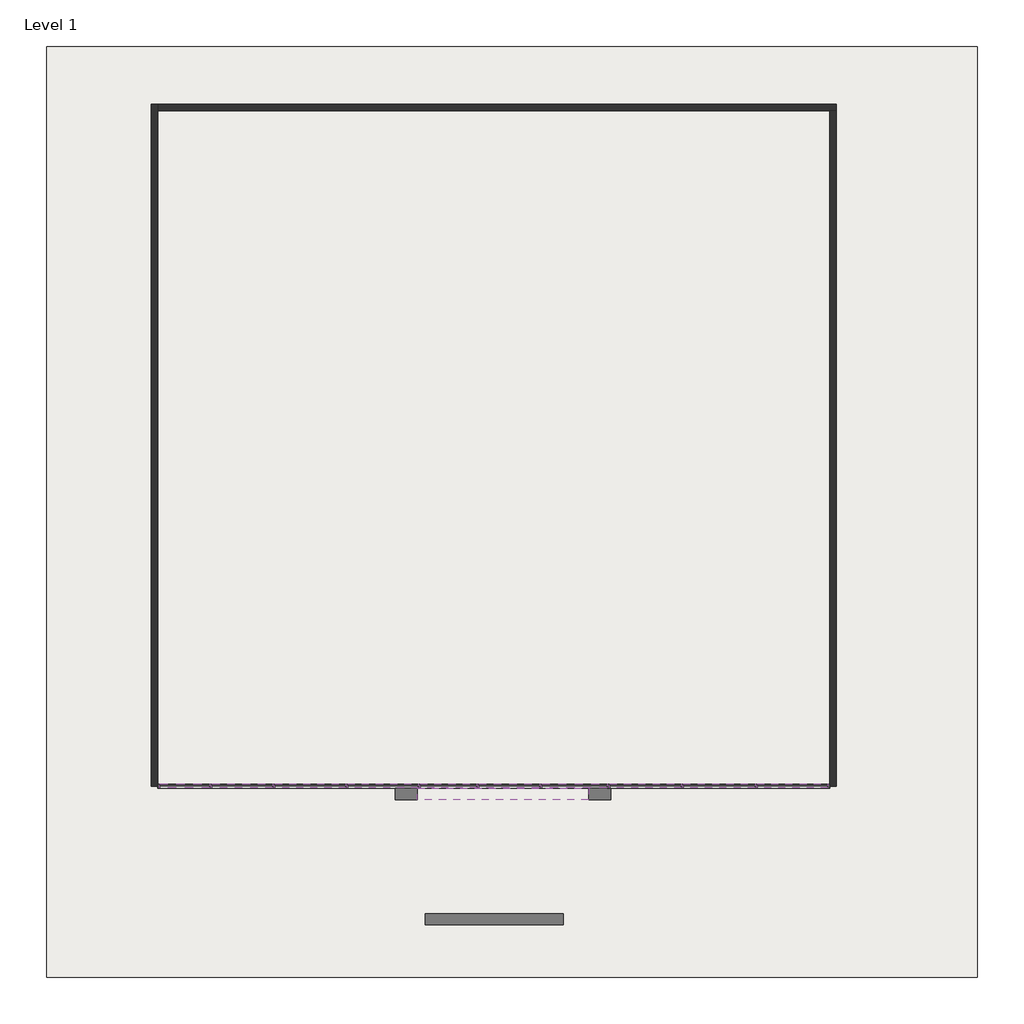
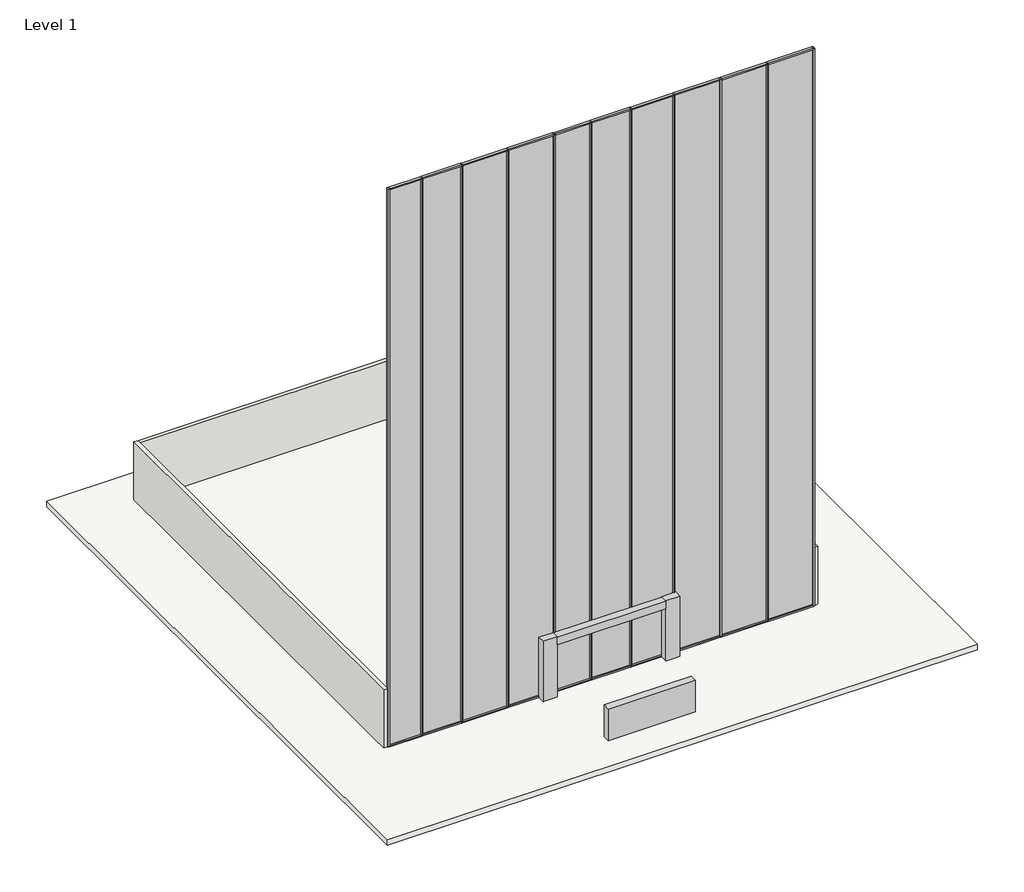
# One storey: 31 members, 10 plates, 3 proxies, 3 walls, 1 slab.
"""IFC4 building model written with IfcOpenShell, lengths in millimetres."""

from ifc_helpers import new_model, si_unit, frame, origin, origin_with_axes, place, context, project, spatial, polyline, outline, extrude, faceted_brep, transform, mapped, element, save
from components import generic_models_17_generic_models_17_a4f02c47, generic_models_2_generic_models_2_43715522, generic_models_3_generic_models_3_4fdafdf2, member_e6c67f36, member_247435d8, member_4a4c44fd, member_995c57f6, member_5c0bf374, member_6d5c3e5e, member_760f9554, member_d9e57c59, member_94459976, system_panel_glazed_c7023cb4, system_panel_glazed_978fe6fd, system_panel_glazed_8ddfe979, system_panel_glazed_c868bc05, system_panel_glazed_b656db30, system_panel_glazed_cc704f4b, system_panel_glazed_e0938204

model = new_model("IFC4")

# Units and contexts
model_context = context("Model", 3, world=origin())
ifc_project = project(units=[si_unit("LENGTHUNIT", "METRE", prefix="MILLI")], contexts=[model_context])

# Site, building, storey
site = spatial("IfcSite", under=ifc_project)
building = spatial("IfcBuilding", under=site)
storey = spatial("IfcBuildingStorey", under=building, Name="Level 1", Elevation=0.0)

# Proxies
placement = place(None, origin())
generic_models_17_generic_models_17_shape = generic_models_17_generic_models_17_a4f02c47(model_context)
element("IfcBuildingElementProxy", 1, Name="Generic Models 17 : Generic Models 17", ObjectType="Generic Models 17 : Generic Models 17", at=placement, inside=storey, context=model_context, shape_type="MappedRepresentation", body=[
    mapped(generic_models_17_generic_models_17_shape, transform((0.0, 0.0, 0.0), x_axis=(1.0, 0.0, 0.0), y_axis=(0.0, 1.0, 0.0), z_axis=(0.0, 0.0, 1.0))),
])
generic_models_2_generic_models_2_shape = generic_models_2_generic_models_2_43715522(model_context)
element("IfcBuildingElementProxy", 2, Name="Generic Models 2 : Generic Models 2", ObjectType="Generic Models 2 : Generic Models 2", at=placement, inside=storey, context=model_context, shape_type="MappedRepresentation", body=[
    mapped(generic_models_2_generic_models_2_shape, transform((0.0, 0.0, 0.0), x_axis=(1.0, 0.0, 0.0), y_axis=(0.0, 1.0, 0.0), z_axis=(0.0, 0.0, 1.0))),
])
generic_models_3_generic_models_3_shape = generic_models_3_generic_models_3_4fdafdf2(model_context)
element("IfcBuildingElementProxy", 3, Name="Generic Models 3 : Generic Models 3", ObjectType="Generic Models 3 : Generic Models 3", at=placement, inside=storey, context=model_context, shape_type="MappedRepresentation", body=[
    mapped(generic_models_3_generic_models_3_shape, transform((0.0, 0.0, 0.0), x_axis=(1.0, 0.0, 0.0), y_axis=(0.0, 1.0, 0.0), z_axis=(0.0, 0.0, 1.0))),
])

# Members
member_shape = member_e6c67f36(model_context)
element("IfcMember", 4, ObjectType="Rectangular Mullion : 2.5\" x 5\" rectangular", at=placement, inside=storey, context=model_context, shape_type="MappedRepresentation", body=[
    mapped(member_shape, transform((12337.7370151, -3682.5004242, 29260.8), x_axis=(0.0, 0.0, 1.0), y_axis=(0.0, -1.0, 0.0), z_axis=(1.0, 0.0, 0.0))),
])
member_2_shape = member_247435d8(model_context)
element("IfcMember", 5, ObjectType="Rectangular Mullion : 2.5\" x 5\" rectangular", at=placement, inside=storey, context=model_context, shape_type="MappedRepresentation", body=[
    mapped(member_2_shape, transform((-8668.0629849, -3682.5004242, 0.0), x_axis=(0.0, 0.0, -1.0), y_axis=(0.0, -1.0, 0.0), z_axis=(-1.0, 0.0, 0.0))),
])
member_3_shape = member_4a4c44fd(model_context)
element("IfcMember", 6, ObjectType="Rectangular Mullion : 2.5\" x 5\" rectangular", at=placement, inside=storey, context=model_context, shape_type="MappedRepresentation", body=[
    mapped(member_3_shape, transform((-7055.1629849, -3682.5004242, 0.0), x_axis=(1.0, 0.0, 0.0), y_axis=(0.0, -1.0, 0.0), z_axis=(0.0, 0.0, -1.0))),
])
element("IfcMember", 7, ObjectType="Rectangular Mullion : 2.5\" x 5\" rectangular", at=placement, inside=storey, context=model_context, shape_type="MappedRepresentation", body=[
    mapped(member_3_shape, transform((-5073.9629849, -3682.5004242, 0.0), x_axis=(1.0, 0.0, 0.0), y_axis=(0.0, -1.0, 0.0), z_axis=(0.0, 0.0, -1.0))),
])
element("IfcMember", 8, ObjectType="Rectangular Mullion : 2.5\" x 5\" rectangular", at=placement, inside=storey, context=model_context, shape_type="MappedRepresentation", body=[
    mapped(member_3_shape, transform((-2787.9629849, -3682.5004242, 0.0), x_axis=(1.0, 0.0, 0.0), y_axis=(0.0, -1.0, 0.0), z_axis=(0.0, 0.0, -1.0))),
])
element("IfcMember", 9, ObjectType="Rectangular Mullion : 2.5\" x 5\" rectangular", at=placement, inside=storey, context=model_context, shape_type="MappedRepresentation", body=[
    mapped(member_3_shape, transform((-501.9629849, -3682.5004242, 0.0), x_axis=(1.0, 0.0, 0.0), y_axis=(0.0, -1.0, 0.0), z_axis=(0.0, 0.0, -1.0))),
])
element("IfcMember", 10, ObjectType="Rectangular Mullion : 2.5\" x 5\" rectangular", at=placement, inside=storey, context=model_context, shape_type="MappedRepresentation", body=[
    mapped(member_3_shape, transform((1326.8370151, -3682.5004242, 0.0), x_axis=(1.0, 0.0, 0.0), y_axis=(0.0, -1.0, 0.0), z_axis=(0.0, 0.0, -1.0))),
])
element("IfcMember", 11, ObjectType="Rectangular Mullion : 2.5\" x 5\" rectangular", at=placement, inside=storey, context=model_context, shape_type="MappedRepresentation", body=[
    mapped(member_3_shape, transform((3308.0370151, -3682.5004242, 0.0), x_axis=(1.0, 0.0, 0.0), y_axis=(0.0, -1.0, 0.0), z_axis=(0.0, 0.0, -1.0))),
])
element("IfcMember", 12, ObjectType="Rectangular Mullion : 2.5\" x 5\" rectangular", at=placement, inside=storey, context=model_context, shape_type="MappedRepresentation", body=[
    mapped(member_3_shape, transform((5441.6370151, -3682.5004242, 0.0), x_axis=(1.0, 0.0, 0.0), y_axis=(0.0, -1.0, 0.0), z_axis=(0.0, 0.0, -1.0))),
])
element("IfcMember", 13, ObjectType="Rectangular Mullion : 2.5\" x 5\" rectangular", at=placement, inside=storey, context=model_context, shape_type="MappedRepresentation", body=[
    mapped(member_3_shape, transform((7761.5036818, -3682.5004242, 0.0), x_axis=(1.0, 0.0, 0.0), y_axis=(0.0, -1.0, 0.0), z_axis=(0.0, 0.0, -1.0))),
])
element("IfcMember", 14, ObjectType="Rectangular Mullion : 2.5\" x 5\" rectangular", at=placement, inside=storey, context=model_context, shape_type="MappedRepresentation", body=[
    mapped(member_3_shape, transform((10081.3703484, -3682.5004242, 0.0), x_axis=(1.0, 0.0, 0.0), y_axis=(0.0, -1.0, 0.0), z_axis=(0.0, 0.0, -1.0))),
])
member_4_shape = member_995c57f6(model_context)
element("IfcMember", 15, ObjectType="Rectangular Mullion : 2.5\" x 5\" rectangular", at=placement, inside=storey, context=model_context, shape_type="MappedRepresentation", body=[
    mapped(member_4_shape, transform((-7023.4129849, -3682.5004242, 0.0), x_axis=(0.0, 0.0, -1.0), y_axis=(0.0, -1.0, 0.0), z_axis=(-1.0, 0.0, 0.0))),
])
element("IfcMember", 16, ObjectType="Rectangular Mullion : 2.5\" x 5\" rectangular", at=placement, inside=storey, context=model_context, shape_type="MappedRepresentation", body=[
    mapped(member_4_shape, transform((1358.5870151, -3682.5004242, 0.0), x_axis=(0.0, 0.0, -1.0), y_axis=(0.0, -1.0, 0.0), z_axis=(-1.0, 0.0, 0.0))),
])
member_5_shape = member_5c0bf374(model_context)
element("IfcMember", 17, ObjectType="Rectangular Mullion : 2.5\" x 5\" rectangular", at=placement, inside=storey, context=model_context, shape_type="MappedRepresentation", body=[
    mapped(member_5_shape, transform((-5042.2129849, -3682.5004242, 0.0), x_axis=(0.0, 0.0, -1.0), y_axis=(0.0, -1.0, 0.0), z_axis=(-1.0, 0.0, 0.0))),
])
element("IfcMember", 18, ObjectType="Rectangular Mullion : 2.5\" x 5\" rectangular", at=placement, inside=storey, context=model_context, shape_type="MappedRepresentation", body=[
    mapped(member_5_shape, transform((-2756.2129849, -3682.5004242, 0.0), x_axis=(0.0, 0.0, -1.0), y_axis=(0.0, -1.0, 0.0), z_axis=(-1.0, 0.0, 0.0))),
])
member_6_shape = member_6d5c3e5e(model_context)
element("IfcMember", 19, ObjectType="Rectangular Mullion : 2.5\" x 5\" rectangular", at=placement, inside=storey, context=model_context, shape_type="MappedRepresentation", body=[
    mapped(member_6_shape, transform((-470.2129849, -3682.5004242, 0.0), x_axis=(0.0, 0.0, -1.0), y_axis=(0.0, -1.0, 0.0), z_axis=(-1.0, 0.0, 0.0))),
])
member_7_shape = member_760f9554(model_context)
element("IfcMember", 20, ObjectType="Rectangular Mullion : 2.5\" x 5\" rectangular", at=placement, inside=storey, context=model_context, shape_type="MappedRepresentation", body=[
    mapped(member_7_shape, transform((3339.7870151, -3682.5004242, 0.0), x_axis=(0.0, 0.0, -1.0), y_axis=(0.0, -1.0, 0.0), z_axis=(-1.0, 0.0, 0.0))),
])
member_8_shape = member_d9e57c59(model_context)
element("IfcMember", 21, ObjectType="Rectangular Mullion : 2.5\" x 5\" rectangular", at=placement, inside=storey, context=model_context, shape_type="MappedRepresentation", body=[
    mapped(member_8_shape, transform((5473.3870151, -3682.5004242, 0.0), x_axis=(0.0, 0.0, -1.0), y_axis=(0.0, -1.0, 0.0), z_axis=(-1.0, 0.0, 0.0))),
])
element("IfcMember", 22, ObjectType="Rectangular Mullion : 2.5\" x 5\" rectangular", at=placement, inside=storey, context=model_context, shape_type="MappedRepresentation", body=[
    mapped(member_8_shape, transform((7793.2536818, -3682.5004242, 0.0), x_axis=(0.0, 0.0, -1.0), y_axis=(0.0, -1.0, 0.0), z_axis=(-1.0, 0.0, 0.0))),
])
element("IfcMember", 23, ObjectType="Rectangular Mullion : 2.5\" x 5\" rectangular", at=placement, inside=storey, context=model_context, shape_type="MappedRepresentation", body=[
    mapped(member_shape, transform((10113.1203484, -3682.5004242, 0.0), x_axis=(0.0, 0.0, -1.0), y_axis=(0.0, -1.0, 0.0), z_axis=(-1.0, 0.0, 0.0))),
])
element("IfcMember", 24, ObjectType="Rectangular Mullion : 2.5\" x 5\" rectangular", at=placement, inside=storey, context=model_context, shape_type="MappedRepresentation", body=[
    mapped(member_2_shape, transform((-7086.9129849, -3682.5004242, 29260.8), x_axis=(0.0, 0.0, 1.0), y_axis=(0.0, -1.0, 0.0), z_axis=(1.0, 0.0, 0.0))),
])
element("IfcMember", 25, ObjectType="Rectangular Mullion : 2.5\" x 5\" rectangular", at=placement, inside=storey, context=model_context, shape_type="MappedRepresentation", body=[
    mapped(member_4_shape, transform((-5105.7129849, -3682.5004242, 29260.8), x_axis=(0.0, 0.0, 1.0), y_axis=(0.0, -1.0, 0.0), z_axis=(1.0, 0.0, 0.0))),
])
element("IfcMember", 26, ObjectType="Rectangular Mullion : 2.5\" x 5\" rectangular", at=placement, inside=storey, context=model_context, shape_type="MappedRepresentation", body=[
    mapped(member_4_shape, transform((3276.2870151, -3682.5004242, 29260.8), x_axis=(0.0, 0.0, 1.0), y_axis=(0.0, -1.0, 0.0), z_axis=(1.0, 0.0, 0.0))),
])
element("IfcMember", 27, ObjectType="Rectangular Mullion : 2.5\" x 5\" rectangular", at=placement, inside=storey, context=model_context, shape_type="MappedRepresentation", body=[
    mapped(member_5_shape, transform((-2819.7129849, -3682.5004242, 29260.8), x_axis=(0.0, 0.0, 1.0), y_axis=(0.0, -1.0, 0.0), z_axis=(1.0, 0.0, 0.0))),
])
element("IfcMember", 28, ObjectType="Rectangular Mullion : 2.5\" x 5\" rectangular", at=placement, inside=storey, context=model_context, shape_type="MappedRepresentation", body=[
    mapped(member_5_shape, transform((-533.7129849, -3682.5004242, 29260.8), x_axis=(0.0, 0.0, 1.0), y_axis=(0.0, -1.0, 0.0), z_axis=(1.0, 0.0, 0.0))),
])
element("IfcMember", 29, ObjectType="Rectangular Mullion : 2.5\" x 5\" rectangular", at=placement, inside=storey, context=model_context, shape_type="MappedRepresentation", body=[
    mapped(member_6_shape, transform((1295.0870151, -3682.5004242, 29260.8), x_axis=(0.0, 0.0, 1.0), y_axis=(0.0, -1.0, 0.0), z_axis=(1.0, 0.0, 0.0))),
])
element("IfcMember", 30, ObjectType="Rectangular Mullion : 2.5\" x 5\" rectangular", at=placement, inside=storey, context=model_context, shape_type="MappedRepresentation", body=[
    mapped(member_7_shape, transform((5409.8870151, -3682.5004242, 29260.8), x_axis=(0.0, 0.0, 1.0), y_axis=(0.0, -1.0, 0.0), z_axis=(1.0, 0.0, 0.0))),
])
element("IfcMember", 31, ObjectType="Rectangular Mullion : 2.5\" x 5\" rectangular", at=placement, inside=storey, context=model_context, shape_type="MappedRepresentation", body=[
    mapped(member_8_shape, transform((7729.7536818, -3682.5004242, 29260.8), x_axis=(0.0, 0.0, 1.0), y_axis=(0.0, -1.0, 0.0), z_axis=(1.0, 0.0, 0.0))),
])
element("IfcMember", 32, ObjectType="Rectangular Mullion : 2.5\" x 5\" rectangular", at=placement, inside=storey, context=model_context, shape_type="MappedRepresentation", body=[
    mapped(member_8_shape, transform((10049.6203484, -3682.5004242, 29260.8), x_axis=(0.0, 0.0, 1.0), y_axis=(0.0, -1.0, 0.0), z_axis=(1.0, 0.0, 0.0))),
])
member_9_shape = member_94459976(model_context)
element("IfcMember", 33, ObjectType="Rectangular Mullion : 2.5\" x 5\" rectangular", at=placement, inside=storey, context=model_context, shape_type="MappedRepresentation", body=[
    mapped(member_9_shape, transform((-8731.5629849, -3682.5004242, 29260.8), x_axis=(-1.0, 0.0, 0.0), y_axis=(0.0, -1.0, 0.0), z_axis=(0.0, 0.0, 1.0))),
])
element("IfcMember", 34, ObjectType="Rectangular Mullion : 2.5\" x 5\" rectangular", at=placement, inside=storey, context=model_context, shape_type="MappedRepresentation", body=[
    mapped(member_9_shape, transform((12401.2370151, -3682.5004242, 0.0), x_axis=(1.0, 0.0, 0.0), y_axis=(0.0, -1.0, 0.0), z_axis=(0.0, 0.0, -1.0))),
])

# Plates
system_panel_glazed_shape = system_panel_glazed_c7023cb4(model_context)
element("IfcPlate", 35, ObjectType="System Panel : Glazed", at=placement, inside=storey, context=model_context, shape_type="MappedRepresentation", body=[
    mapped(system_panel_glazed_shape, transform((-7877.4879849, -3682.5004242, 63.5), x_axis=(1.0, 0.0, 0.0), y_axis=(0.0, 1.0, 0.0), z_axis=(0.0, 0.0, 1.0))),
])
system_panel_glazed_2_shape = system_panel_glazed_978fe6fd(model_context)
element("IfcPlate", 36, ObjectType="System Panel : Glazed", at=placement, inside=storey, context=model_context, shape_type="MappedRepresentation", body=[
    mapped(system_panel_glazed_2_shape, transform((-6064.5629849, -3682.5004242, 63.5), x_axis=(1.0, 0.0, 0.0), y_axis=(0.0, 1.0, 0.0), z_axis=(0.0, 0.0, 1.0))),
])
element("IfcPlate", 37, ObjectType="System Panel : Glazed", at=placement, inside=storey, context=model_context, shape_type="MappedRepresentation", body=[
    mapped(system_panel_glazed_2_shape, transform((2317.4370151, -3682.5004242, 63.5), x_axis=(1.0, 0.0, 0.0), y_axis=(0.0, 1.0, 0.0), z_axis=(0.0, 0.0, 1.0))),
])
system_panel_glazed_3_shape = system_panel_glazed_8ddfe979(model_context)
element("IfcPlate", 38, ObjectType="System Panel : Glazed", at=placement, inside=storey, context=model_context, shape_type="MappedRepresentation", body=[
    mapped(system_panel_glazed_3_shape, transform((-3930.9629849, -3682.5004242, 63.5), x_axis=(1.0, 0.0, 0.0), y_axis=(0.0, 1.0, 0.0), z_axis=(0.0, 0.0, 1.0))),
])
element("IfcPlate", 39, ObjectType="System Panel : Glazed", at=placement, inside=storey, context=model_context, shape_type="MappedRepresentation", body=[
    mapped(system_panel_glazed_3_shape, transform((-1644.9629849, -3682.5004242, 63.5), x_axis=(1.0, 0.0, 0.0), y_axis=(0.0, 1.0, 0.0), z_axis=(0.0, 0.0, 1.0))),
])
system_panel_glazed_4_shape = system_panel_glazed_c868bc05(model_context)
element("IfcPlate", 40, ObjectType="System Panel : Glazed", at=placement, inside=storey, context=model_context, shape_type="MappedRepresentation", body=[
    mapped(system_panel_glazed_4_shape, transform((412.4370151, -3682.5004242, 63.5), x_axis=(1.0, 0.0, 0.0), y_axis=(0.0, 1.0, 0.0), z_axis=(0.0, 0.0, 1.0))),
])
system_panel_glazed_5_shape = system_panel_glazed_b656db30(model_context)
element("IfcPlate", 41, ObjectType="System Panel : Glazed", at=placement, inside=storey, context=model_context, shape_type="MappedRepresentation", body=[
    mapped(system_panel_glazed_5_shape, transform((4374.8370151, -3682.5004242, 63.5), x_axis=(1.0, 0.0, 0.0), y_axis=(0.0, 1.0, 0.0), z_axis=(0.0, 0.0, 1.0))),
])
system_panel_glazed_6_shape = system_panel_glazed_cc704f4b(model_context)
element("IfcPlate", 42, ObjectType="System Panel : Glazed", at=placement, inside=storey, context=model_context, shape_type="MappedRepresentation", body=[
    mapped(system_panel_glazed_6_shape, transform((6601.5703484, -3682.5004242, 63.5), x_axis=(1.0, 0.0, 0.0), y_axis=(0.0, 1.0, 0.0), z_axis=(0.0, 0.0, 1.0))),
])
element("IfcPlate", 43, ObjectType="System Panel : Glazed", at=placement, inside=storey, context=model_context, shape_type="MappedRepresentation", body=[
    mapped(system_panel_glazed_6_shape, transform((8921.4370151, -3682.5004242, 63.5), x_axis=(1.0, 0.0, 0.0), y_axis=(0.0, 1.0, 0.0), z_axis=(0.0, 0.0, 1.0))),
])
system_panel_glazed_7_shape = system_panel_glazed_e0938204(model_context)
element("IfcPlate", 44, ObjectType="System Panel : Glazed", at=placement, inside=storey, context=model_context, shape_type="MappedRepresentation", body=[
    mapped(system_panel_glazed_7_shape, transform((11225.4286818, -3682.5004242, 63.5), x_axis=(1.0, 0.0, 0.0), y_axis=(0.0, 1.0, 0.0), z_axis=(0.0, 0.0, 1.0))),
])

# Slab
element("IfcSlab", 45, ObjectType="Generic - 12\"", at=placement, inside=storey, context=model_context, shape_type="SweptSolid", body=[
    extrude(outline(polyline([(17039.0583051, 19564.8726593), (17039.0583051, -9695.9273407), (-12221.7416949, -9695.9273407), (-12221.7416949, 19564.8726593), (17039.0583051, 19564.8726593)])), frame((0.0, 0.0, -304.8), z_axis=(0.0, 0.0, 1.0), x_axis=(1.0, 0.0, 0.0)), (0.0, 0.0, 1.0), 304.8),
])

# Walls
element("IfcWall", 46, ObjectType="outer wall", at=placement, inside=storey, context=model_context, shape_type="Brep", body=[
    faceted_brep([(-8731.5629849, -3682.5004242, 0.0), (-8731.5629849, 17551.8995758, 0.0), (-8731.5629849, 17755.0995758, 0.0), (-8731.5629849, 17755.0995758, 3048.0), (-8731.5629849, 17551.8995758, 3048.0), (-8731.5629849, -3682.5004242, 3048.0), (-8934.7629849, -3682.5004242, 0.0), (-8934.7629849, -3682.5004242, 3048.0), (-8934.7629849, 17551.8995758, 3048.0), (-8934.7629849, 17755.0995758, 3048.0), (-8934.7629849, 17755.0995758, 0.0)], [[[0, 1, 2, 3, 4, 5]], [[6, 7, 8, 9, 10]], [[2, 1, 0, 6, 10]], [[0, 5, 7, 6]], [[5, 4, 3, 9, 8, 7]], [[3, 2, 10, 9]]]),
])
element("IfcWall", 47, ObjectType="outer wall", at=placement, inside=storey, context=model_context, shape_type="Brep", body=[
    faceted_brep([(-8731.5629849, 17551.8995758, 3048.0), (-8731.5629849, 17551.8995758, 0.0), (12401.2370151, 17551.8995758, 0.0), (12604.4370151, 17551.8995758, 0.0), (12604.4370151, 17551.8995758, 3048.0), (12401.2370151, 17551.8995758, 3048.0), (-8731.5629849, 17755.0995758, 0.0), (-8731.5629849, 17755.0995758, 3048.0), (12604.4370151, 17755.0995758, 3048.0), (12604.4370151, 17755.0995758, 0.0)], [[[0, 1, 2, 3, 4, 5]], [[6, 7, 8, 9]], [[3, 2, 1, 6, 9]], [[0, 5, 4, 8, 7]], [[0, 7, 6, 1]], [[4, 3, 9, 8]]]),
])
element("IfcWall", 48, ObjectType="outer wall", at=placement, inside=storey, context=model_context, shape_type="SweptSolid", body=[
    extrude(outline(polyline([(12401.2370151, -3682.5004242), (12401.2370151, 17551.8995758), (12604.4370151, 17551.8995758), (12604.4370151, -3682.5004242), (12401.2370151, -3682.5004242)])), origin_with_axes(), (0.0, 0.0, 1.0), 3048.0),
])

save(model, "model.ifc")

# Revit data of these elements
# Type "Rectangular Mullion : 2.5\" x 5\" rectangular"
#   built-in parameter 1007304 = 0.416667 (stored number, unit not read)
#   built-in parameter 1007301 = 0.104167 (stored number, unit not read)
#   built-in parameter 1007300 = 0.104167 (stored number, unit not read)
# Type "System Panel : Glazed"
#   Construction Type Id = "GSP4R"
#   Analytic Construction = "1/8 in Pilkington single glazing"
#   Visual Light Transmittance = 0.9
#   Solar Heat Gain Coefficient = 0.86
#   Heat Transfer Coefficient (U) = 1.18115 BTU/(h·ft²·°F)
# Type "Generic - 12\""
#   Assembly Code = "B1010"
#   Function = 0
#   Layers, outside or top first: 1' - 0" no material (function 1)
# Type "outer wall"
#   Assembly Code = "B2010"
#   Layers, outside or top first: 0' - 8" "Copper" (function 1)
# Element 1 (IfcBuildingElementProxy, "Generic Models 17 : Generic Models 17")
#   Phase Created = New Construction
# Element 2 (IfcBuildingElementProxy, "Generic Models 2 : Generic Models 2")
#   Phase Created = New Construction
# Element 3 (IfcBuildingElementProxy, "Generic Models 3 : Generic Models 3")
#   Phase Created = New Construction
# Elements 4, 5, 6, 7, 8, 9, 10, 11, 12, 13, 14, 15, 16, 17, 18, 19, 20, 21, 22, 23, 24, 25, 26, 27, 28, 29, 30, 31, 32, 33, 34 (IfcMember, "Rectangular Mullion : 2.5\" x 5\" rectangular")
#   Phase Created = New Construction
#   Materials on its faces: "Aluminum"
# Elements 35, 36, 37, 38, 39, 40, 41, 42, 43, 44 (IfcPlate, "System Panel : Glazed")
#   Phase Created = New Construction
#   Materials on its faces: "Glass"
# Element 45 (IfcSlab, "Generic - 12\"")
#   Height Offset From Level = 0' - 0"
#   Phase Created = New Construction
#   Materials on its faces: "Default Floor"
# Elements 46, 47, 48 (IfcWall, "outer wall")
#   Top Offset = 0' - 0"
#   Base Offset = 0' - 0"
#   Unconnected Height = 96' - 0"
#   wall height = 96' - 0"
#   Phase Created = New Construction
#   Base Constraint = Level 1
#   Materials on its faces: "Copper"
# Materials
#   "Copper": class "Metal", colour RGB 0 0 0, transparency 0, Description = "Copper, matte finish", Cost = 0
#   "Aluminum": class "Metal", colour RGB 247 247 247, transparency 0, Description = "Aluminum 6061", Cost = 0
#   "Glass": class "Glass", colour RGB 0 128 192, transparency 0.75, Description = "Soda Lime Glass", Cost = 0
#   "Default Floor": colour RGB 128 128 128, transparency 0
